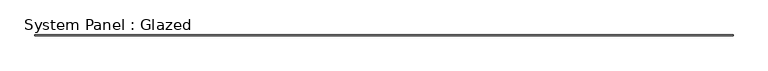
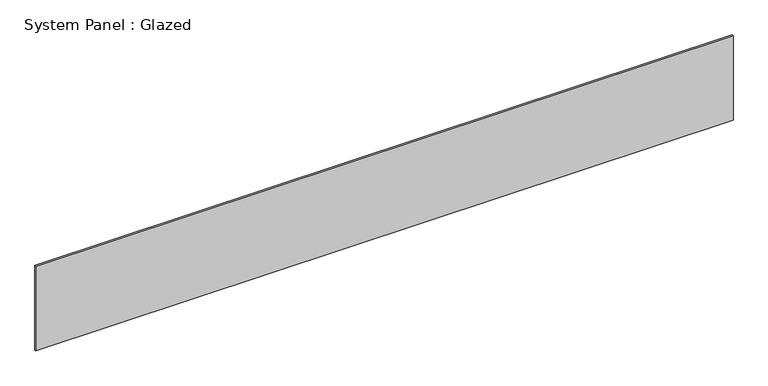
"""IFC4 building model written with IfcOpenShell, lengths in millimetres: plate geometry, System Panel : Glazed."""

from ifc_helpers import new_model, si_unit, origin, origin_with_axes, place, context, project, spatial, polyline, outline, extrude, source, transform, mapped, element, save


def system_panel_glazed_6867f845(model_context):
    return source(origin(), model_context, "Body", "SweptSolid", [
        extrude(outline(polyline([(8305.8, 19.05), (-8305.8, 19.05), (-8305.8, 44.45), (8305.8, 44.45), (8305.8, 19.05)])), origin_with_axes(), (0.0, 0.0, 1.0), 2133.6),
    ])


if __name__ == "__main__":
    model = new_model("IFC4")
    model_context = context("Model", 3, world=origin())
    ifc_project = project(units=[si_unit("LENGTHUNIT", "METRE", prefix="MILLI")], contexts=[model_context])
    site = spatial("IfcSite", under=ifc_project)
    building = spatial("IfcBuilding", under=site)
    placement = place(None, origin())
    system_panel_glazed_shape = system_panel_glazed_6867f845(model_context)
    element("IfcPlate", 1, ObjectType="System Panel : Glazed", at=placement, inside=building, context=model_context, shape_type="MappedRepresentation", body=[
        mapped(system_panel_glazed_shape, transform((0.0, 0.0, 0.0), x_axis=(1.0, 0.0, 0.0), y_axis=(0.0, 1.0, 0.0), z_axis=(0.0, 0.0, 1.0))),
    ])
    save(model, "model.ifc")

# Revit data of these elements
# Type "System Panel : Glazed"
#   Construction Type Id = "GSP4R"
#   Analytic Construction = "1/8 in Pilkington single glazing"
#   Visual Light Transmittance = 0.9
#   Solar Heat Gain Coefficient = 0.86
#   Heat Transfer Coefficient (U) = 1.18115 BTU/(h·ft²·°F)
# Element 1 (IfcPlate, "System Panel : Glazed")
#   Materials on its faces: "Glass"
# Materials
#   "Glass": class "Glass", colour RGB 0 128 192, transparency 0.75, Description = "Soda Lime Glass", Cost = 0
